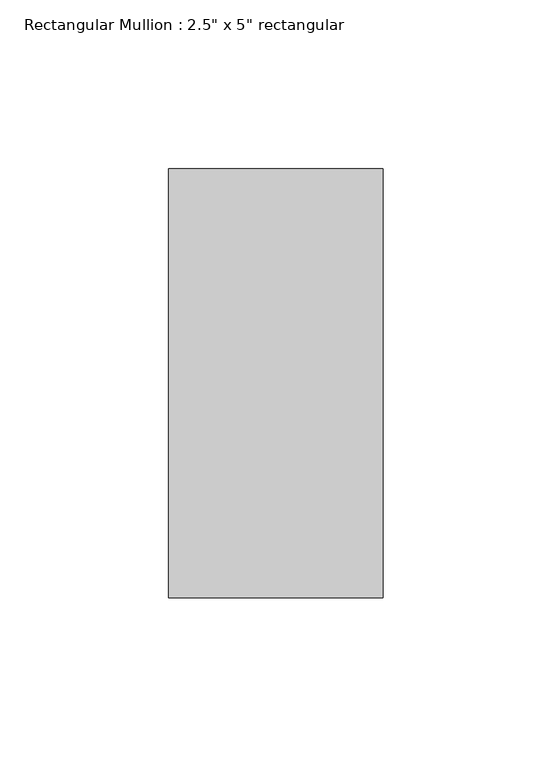
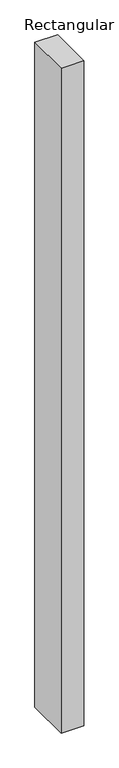
"""IFC4 building model written with IfcOpenShell, lengths in millimetres: member geometry."""

from ifc_helpers import new_model, si_unit, frame, origin, place, context, project, spatial, polyline, outline, extrude, source, transform, mapped, element, save


def member_3112dcca(model_context):
    return source(origin(), model_context, "Body", "SweptSolid", [
        extrude(outline(polyline([(31.75, 63.5), (31.75, -63.5), (-31.75, -63.5), (-31.75, 63.5), (31.75, 63.5)])), frame((0.0, 0.0, -1970.8332834), z_axis=(0.0, 0.0, 1.0), x_axis=(1.0, 0.0, 0.0)), (0.0, 0.0, 1.0), 1970.8332834),
    ])


if __name__ == "__main__":
    model = new_model("IFC4")
    model_context = context("Model", 3, world=origin())
    ifc_project = project(units=[si_unit("LENGTHUNIT", "METRE", prefix="MILLI")], contexts=[model_context])
    site = spatial("IfcSite", under=ifc_project)
    building = spatial("IfcBuilding", under=site)
    placement = place(None, origin())
    member_shape = member_3112dcca(model_context)
    element("IfcMember", 1, ObjectType="Rectangular Mullion : 2.5\" x 5\" rectangular", at=placement, inside=building, context=model_context, shape_type="MappedRepresentation", body=[
        mapped(member_shape, transform((0.0, 0.0, 0.0), x_axis=(1.0, 0.0, 0.0), y_axis=(0.0, 1.0, 0.0), z_axis=(0.0, 0.0, 1.0))),
    ])
    save(model, "model.ifc")

# Revit data of these elements
# Type "Rectangular Mullion : 2.5\" x 5\" rectangular"
#   built-in parameter 1007304 = 0.416667 (stored number, unit not read)
#   built-in parameter 1007301 = 0.104167 (stored number, unit not read)
#   built-in parameter 1007300 = 0.104167 (stored number, unit not read)
# Element 1 (IfcMember, "Rectangular Mullion : 2.5\" x 5\" rectangular")
#   Materials on its faces: "Aluminum"
# Materials
#   "Aluminum": class "Metal", colour RGB 247 247 247, transparency 0, Description = "Aluminum 6061", Cost = 0
